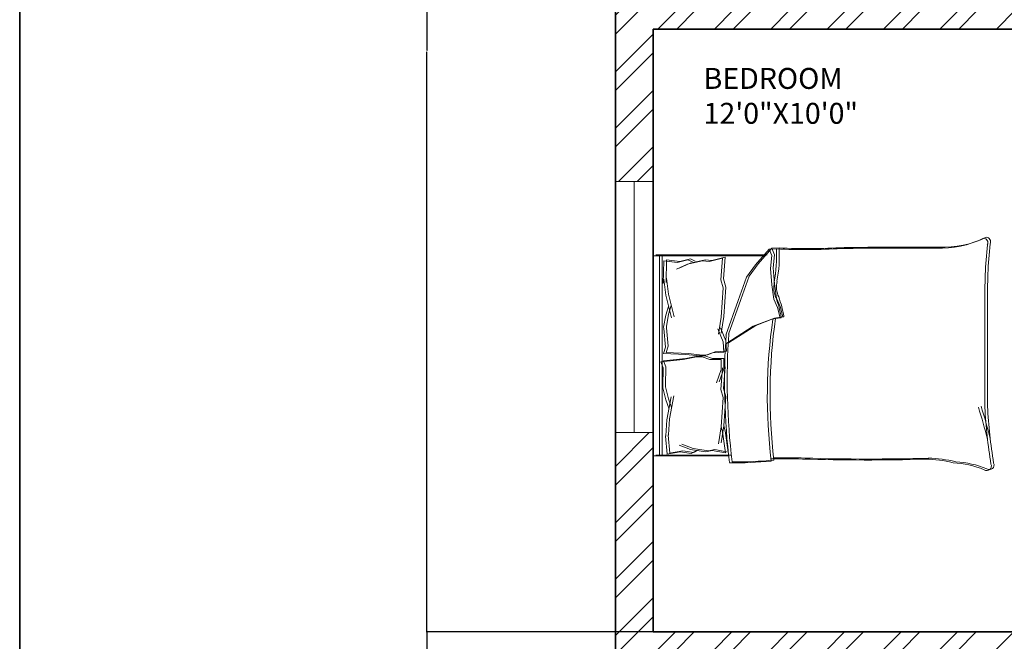
# Model space of a CAD drawing. Units: inches. Extents: x 2120 to 4013, y 1390 to 3019.
# Tile 28 of 59: x 2120 to 2356, y 2073 to 2221. Entities that reach past the tile are written whole.
import ezdxf

# ---------------------------------------------------------------- set-up
doc = ezdxf.new("R2010")
doc.units = ezdxf.units.IN
for name, color, linetype, lineweight in [('A-ANNO-DIMS', 2, 'Continuous', 18), ('A-ANNO-TTLB', 7, 'Continuous', 35), ('A-AREA-IDEN', 7, 'Continuous', 18), ('A-FURN', 8, 'Continuous', 13), ('A-GLAZ', 4, 'Continuous', 18), ('A-WALL', 7, 'Continuous', 35), ('A-WALL-PATT', 252, 'Continuous', 13)]:
    doc.layers.add(name, color=color, linetype=linetype, lineweight=lineweight)
doc.styles.get("Standard").update_dxf_attribs({"font": 'arial.ttf'})
doc.dimstyles.get("Standard").update_dxf_attribs({"dimtxt": 0.18, "dimasz": 0.18, "dimexe": 0.18, "dimexo": 0.0625, "dimgap": 0.09, "dimtad": 0, "dimtih": 1, "dimtoh": 1, "dimdec": 4, "dimzin": 0, "dimdsep": 46, "dimtxsty": 'Standard', "dimcen": 0.09, "dimadec": 0, "dimazin": 0, "dimtfac": 1, "dimtdec": 4, "dimtofl": 0, "dimtmove": 0, "dimatfit": 3, "dimfxl": 1, "dimtolj": 1, "dimtzin": 0, "dimarcsym": 0})

# ---------------------------------------------------------------- blocks, each defined once
blk = doc.blocks.new('BED-DOUBLE-PLAN')
for p, q in [((3.48, 63.34), (3.48, 81.45)), ((3.48, 81.45), (51.27, 81.45)), ((3.7, 62.7), (3.7, 80.81)), ((51.27, 81.45), (51.27, 54.84)), ((51.5, 80.81), (51.5, 54.2)), ((3.48, 79.91), (51.27, 79.91)), ((3.7, 79.27), (51.5, 79.27)), ((3.9, 78.11), (8.18, 78.44)), ((3.9, 78.13), (4.47, 74.95)), ((4.13, 77.47), (8.41, 77.8)), ((8.18, 78.44), (8.29, 78.42)), ((8.29, 78.42), (12.11, 78.13)), ((8.41, 77.8), (8.51, 77.78)), ((8.51, 77.78), (12.34, 77.49)), ((12.11, 78.13), (17.6, 77.12)), ((14.86, 77.7), (16.88, 78.42)), ((15.08, 77.06), (17.11, 77.78)), ((16.88, 78.42), (19.77, 79.14)), ((17.11, 77.78), (20, 78.5)), ((19.77, 79.14), (20.09, 79.14)), ((20, 78.5), (20.32, 78.5)), ((20.09, 79.14), (24.54, 79)), ((20.32, 78.5), (24.77, 78.36)), ((24.54, 79), (25.98, 79.58)), ((24.77, 78.36), (26.21, 78.94)), ((25.98, 79.58), (26.56, 74.23)), ((26.21, 78.94), (26.79, 73.59)), ((27.98, 78.95), (27.73, 73.58)), ((28.21, 78.32), (27.96, 72.94)), ((29.46, 78.47), (27.98, 78.95)), ((29.69, 77.83), (28.21, 78.32)), ((33.89, 78.89), (29.46, 78.47)), ((34.11, 78.25), (29.69, 77.83)), ((34.21, 78.91), (33.89, 78.89)), ((34.43, 78.27), (34.11, 78.25)), ((37.14, 78.37), (34.21, 78.91)), ((37.37, 77.73), (34.43, 78.27)), ((41.92, 78.38), (36.5, 77.02)), ((42.14, 77.74), (36.72, 76.38)), ((39.2, 77.77), (37.14, 78.37)), ((39.43, 77.13), (37.37, 77.73)), ((45.71, 78.9), (41.92, 78.38)), ((45.94, 78.26), (42.14, 77.74)), ((50.11, 78.89), (44.71, 78.99)), ((44.71, 78.99), (45.71, 78.9)), ((50.34, 78.25), (44.94, 78.35)), ((44.94, 78.35), (45.94, 78.26)), ((50.11, 78.89), (49.73, 75.68)), ((50.34, 78.25), (49.96, 75.04)), ((4.12, 77.49), (4.7, 74.31)), ((12.34, 77.49), (17.83, 76.48)), ((49.31, 73.19), (48.13, 75.87)), ((49.73, 75.68), (50.33, 73.11)), ((4.47, 74.95), (4.04, 72.35)), ((4.7, 74.31), (4.27, 71.71)), ((5.05, 72.49), (6.06, 75.24)), ((5.28, 71.85), (6.29, 74.6)), ((26.56, 74.23), (27.14, 71.05)), ((26.79, 73.59), (27.37, 70.41)), ((27.73, 73.58), (27.36, 70.37)), ((27.96, 72.94), (27.58, 69.73)), ((49.54, 72.55), (48.36, 75.23)), ((50.11, 69.62), (49.31, 73.19)), ((50.33, 73.11), (49.82, 72.06)), ((49.96, 75.04), (50.56, 72.47)), ((4.04, 72.35), (4.62, 71.33)), ((4.27, 71.71), (4.85, 70.7)), ((4.47, 68.88), (5.05, 72.49)), ((4.7, 68.24), (5.28, 71.85)), ((27.14, 71.05), (27.14, 69.74)), ((50.34, 68.98), (49.54, 72.55)), ((50.56, 72.47), (50.04, 71.42)), ((4.76, 67.29), (4.47, 68.88)), ((4.99, 66.65), (4.7, 68.24)), ((27.14, 69.74), (26.56, 67.86)), ((27.37, 69.1), (26.79, 67.23)), ((27.36, 70.37), (27.44, 69.07)), ((27.37, 70.41), (27.37, 69.1)), ((27.44, 69.07), (28.13, 67.23)), ((27.58, 69.73), (27.67, 68.43)), ((27.67, 68.43), (28.36, 66.59)), ((49.92, 68.01), (50.11, 69.62)), ((50.15, 67.37), (50.34, 68.98)), ((4.19, 64.11), (4.76, 67.29)), ((4.41, 63.47), (4.99, 66.65)), ((24.1, 65.18), (20.96, 66.27)), ((26.56, 67.86), (26.56, 65.18)), ((26.79, 67.23), (26.79, 64.54)), ((28.13, 67.23), (28.3, 64.55)), ((28.36, 66.59), (28.53, 63.91)), ((30.75, 64.71), (33.82, 65.99)), ((50.7, 64.87), (49.92, 68.01)), ((50.93, 64.23), (50.15, 67.37)), ((9.28, 64.83), (4.19, 64.11)), ((9.51, 64.19), (4.41, 63.47)), ((6.38, 65.82), (10.42, 65.15)), ((6.61, 65.18), (10.64, 64.51)), ((10.42, 65.15), (9.28, 64.83)), ((10.64, 64.51), (9.51, 64.19)), ((10.42, 65.15), (17.43, 64.72)), ((10.64, 64.51), (17.65, 64.08)), ((17.43, 64.72), (19.39, 65.28)), ((17.65, 64.08), (19.61, 64.64)), ((19.39, 65.28), (24.52, 64.87)), ((19.61, 64.64), (24.75, 64.23)), ((24.33, 64.54), (21.19, 65.63)), ((26.56, 65.18), (24.1, 65.18)), ((26.79, 64.54), (24.33, 64.54)), ((28.3, 64.55), (30.75, 64.71)), ((28.53, 63.91), (30.98, 64.07)), ((30.26, 64.06), (34.45, 57.57)), ((30.98, 64.07), (34.05, 65.35)), ((40.65, 61.13), (32.31, 64.06)), ((32.57, 65.82), (36.6, 65.15)), ((32.79, 65.18), (36.83, 64.51)), ((36.6, 65.15), (43.61, 64.72)), ((36.83, 64.51), (43.84, 64.08)), ((43.61, 64.72), (45.57, 65.28)), ((43.84, 64.08), (45.8, 64.64)), ((45.57, 65.28), (50.7, 64.87)), ((45.8, 64.64), (50.93, 64.23)), ((30.49, 63.42), (34.68, 56.93)), ((40.87, 60.49), (32.54, 63.42)), ((46.22, 59.12), (40.65, 61.13)), ((46.45, 58.48), (40.87, 60.49)), ((49.16, 56.95), (46.22, 59.12)), ((34.45, 57.57), (36.15, 53.08)), ((34.68, 56.93), (36.38, 52.44)), ((49.39, 56.31), (46.45, 58.48)), ((52.87, 53.7), (49.16, 56.95)), ((53.1, 53.06), (49.39, 56.31)), ((36.15, 53.08), (36.46, 51.07)), ((36.38, 52.44), (36.69, 50.43)), ((38.94, 51.69), (40.96, 52.62)), ((39.17, 51.05), (41.18, 51.98)), ((40.96, 52.62), (44.36, 53.08)), ((41.18, 51.98), (44.59, 52.44)), ((44.36, 53.08), (48.23, 53.39)), ((44.59, 52.44), (48.46, 52.75)), ((48.23, 53.39), (51.33, 53.08)), ((48.46, 52.75), (51.56, 52.44)), ((51.33, 53.08), (52.87, 53.7)), ((51.56, 52.44), (53.1, 53.06)), ((52.95, 51.96), (52.87, 53.7, 3.87)), ((53.18, 51.32), (53.1, 53.06, 3.87)), ((36.46, 51.07), (38.94, 51.69)), ((36.69, 50.43), (39.17, 51.05)), ((15.06, 2.2), (39.68, 2.2)), ((15.29, 1.56), (39.91, 1.56))]:
    blk.add_line(p, q)
for centre, radius, start, end in [((21.36, -100.61), 164.97, 86.0865, 96.7821), ((21.59, -101.25), 164.97, 86.0865, 96.7821), ((85.16, 61.35), 83.31, 178.7218, 185.604), ((85.39, 60.71), 83.31, 178.7218, 185.604), ((17.76, -74.87), 129.02, 81.7845, 96.9006), ((17.99, -75.51), 129.02, 81.7845, 96.9006), ((-167.31, 50.27), 170.11, 358.4762, 1.0082), ((-167.08, 49.63), 170.11, 358.4762, 1.0082), ((31.16, 79.96), 29.65, 280.6617, 289.8806), ((43.74, 46.38), 6.22, 78.6608, 113.7384), ((43.97, 45.74), 6.22, 78.6608, 113.7384), ((51.33, 88.1), 36.18, 259.8763, 272.5657), ((51.56, 87.46), 36.18, 259.8763, 272.5657), ((182.27, 45.13), 129.5, 176.9791, 183.8365), ((36.64, 51.01), 0.185, 160.2464, 271.1377), ((36.87, 50.37), 0.185, 160.2464, 271.1377), ((31.38, 79.32), 29.65, 280.6617, 289.8806), ((182.5, 44.49), 129.5, 176.9791, 183.8365), ((484.82, 30.83), 482.31, 178.2277, 181.7185), ((485.05, 30.19), 482.31, 178.2277, 181.7185), ((-4508.74, 13.62), 4561.86, 0.00217, 0.28689), ((-4508.51, 12.99), 4561.86, 0.00217, 0.28689), ((-26.9, 16.93), 29.63, 346.0648, 358.9113), ((-26.67, 16.29), 29.63, 346.0648, 358.9113), ((76.16, 12.78), 23.07, 177.4714, 206.4681), ((76.39, 12.14), 23.07, 177.4714, 206.4681), ((-21.66, 11.17), 23.56, 337.9751, 356.652), ((-21.43, 10.53), 23.56, 337.9751, 356.652), ((-17.22, 105.16), 106.46, 283.3832, 287.7053), ((-16.99, 104.52), 106.46, 283.3832, 287.7053), ((54.41, 2.58), 1.1, 242.6588, 356.02), ((1.09, 1.73), 1.09, 146.1736, 293.4781), ((1.32, 1.09), 1.09, 146.1736, 293.4781), ((21.43, -119.39), 121.76, 92.9958, 99.4091), ((21.66, -120.03), 121.76, 92.9958, 99.4091), ((41.15, -130.83), 133.04, 84.4998, 90.6351), ((41.38, -131.47), 133.04, 84.4998, 90.6351), ((54.64, 1.94), 1.1, 242.6588, 356.02)]:
    blk.add_arc(centre, radius, start, end)
blk = doc.blocks.new('WIN-PLAN-60IN')
for p, q in [((0, 9), (0, 0)), ((60, 4.5), (60, 9)), ((60, 9), (60, 0)), ((0, 0), (0, 4.5)), ((0, 4.5), (60, 4.5))]:
    blk.add_line(p, q)
blk = doc.blocks.new('*D214')
at = {"layer": 'A-ANNO-DIMS', "color": 0, "lineweight": -2, "transparency": 16777216}
for p, q in [((2271.67, 2075.03), (2217.55, 2075.03)), ((2217.73, 2074.85), (2217.73, 1970.46)), ((2217.73, 1865.71), (2217.73, 1970.1)), ((2271.67, 1865.53), (2217.55, 1865.53))]:
    blk.add_line(p, q, dxfattribs=at)
at = {"layer": 'A-ANNO-DIMS', "color": 0, "transparency": 16777216}
for points in [[(2217.7, 2074.85), (2217.76, 2074.85), (2217.73, 2075.03)], [(2217.7, 1865.71), (2217.76, 1865.71), (2217.73, 1865.53)]]:
    blk.add_solid(points, dxfattribs=at)
at = {"layer": 'Defpoints', "color": 0, "transparency": 16777216}
for p in [(2217.73, 2075.03), (2271.73, 2075.03), (2271.73, 1865.53)]:
    blk.add_point(p, dxfattribs=at)
at = {"layer": 'A-ANNO-DIMS', "color": 0, "transparency": 16777216, "insert": (2217.73, 1970.28), "char_height": 0.18, "attachment_point": 5}
blk.add_mtext('\\A1;209.5', dxfattribs=at)
blk = doc.blocks.new('*D215')
at = {"layer": 'A-ANNO-DIMS', "color": 0, "lineweight": -2, "transparency": 16777216}
for p, q in [((2262.67, 2352.53), (2217.55, 2352.53)), ((2217.73, 2352.35), (2217.73, 2213.96)), ((2217.73, 2075.21), (2217.73, 2213.6)), ((2271.67, 2075.03), (2217.55, 2075.03))]:
    blk.add_line(p, q, dxfattribs=at)
at = {"layer": 'A-ANNO-DIMS', "color": 0, "transparency": 16777216}
for points in [[(2217.7, 2352.35), (2217.76, 2352.35), (2217.73, 2352.53)], [(2217.7, 2075.21), (2217.76, 2075.21), (2217.73, 2075.03)]]:
    blk.add_solid(points, dxfattribs=at)
at = {"layer": 'Defpoints', "color": 0, "transparency": 16777216}
for p in [(2217.73, 2352.53), (2262.73, 2352.53), (2271.73, 2075.03)]:
    blk.add_point(p, dxfattribs=at)
at = {"layer": 'A-ANNO-DIMS', "color": 0, "transparency": 16777216, "insert": (2217.73, 2213.78), "char_height": 0.18, "attachment_point": 5}
blk.add_mtext('\\A1;277.5', dxfattribs=at)

msp = doc.modelspace()

# ---------------------------------------------------------------- hatches: boundary and pattern name
at = {"layer": 'A-WALL-PATT'}
h = msp.add_hatch(dxfattribs=at)
h.set_pattern_fill('ANSI32', color=256)
h.paths.add_polyline_path([(2271.7331, 2343.531), (2283.3788, 2343.531), (2283.3788, 2348.031), (2283.3788, 2352.5306), (2262.7331, 2352.5306), (2262.7331, 2182.638), (2267.2331, 2182.638), (2271.7331, 2182.638), (2271.7331, 2219.031), (2391.7331, 2219.031), (2391.7331, 2214.189), (2393.9831, 2214.189), (2396.2331, 2214.189), (2396.2331, 2219.031), (2420.2331, 2219.031), (2420.2331, 2225.7535), (2417.2197, 2225.7535), (2415.7331, 2225.7535), (2415.7331, 2223.5306), (2271.7331, 2223.5306)])
h.paths.add_polyline_path([(2380.0942, 2352.5306), (2343.3788, 2352.5306), (2343.3788, 2343.531), (2363.2331, 2343.531), (2363.2331, 2288.8489), (2365.4831, 2288.8489), (2367.7331, 2288.8489), (2367.7331, 2343.531), (2380.0942, 2343.531)], flags=17)
h.paths.add_polyline_path([(2432.4339, 2352.5306), (2404.0943, 2352.5306), (2404.0943, 2343.531), (2415.7331, 2343.531), (2415.7331, 2264.0306), (2367.7331, 2264.0306), (2367.7331, 2266.4872), (2363.2331, 2266.4872), (2363.2331, 2259.531), (2367.7331, 2259.531), (2415.7331, 2259.531), (2415.7331, 2255.0658), (2420.2331, 2255.0658), (2420.2331, 2259.531), (2424.5717, 2259.531), (2424.5717, 2261.781), (2424.5717, 2264.0306), (2420.2331, 2264.0306), (2420.2331, 2343.531), (2432.4339, 2343.531)])
h.paths.add_polyline_path([(2508.9115, 2352.5306), (2456.4339, 2352.5306), (2456.4339, 2343.531), (2468.2331, 2343.531), (2468.2331, 2264.0306), (2448.0487, 2264.0306), (2448.0487, 2259.531), (2468.2331, 2259.531), (2468.2331, 2255.5496), (2472.7331, 2255.5496), (2472.7331, 2343.531), (2508.9115, 2343.531)])
h.paths.add_polyline_path([(2637.7331, 2352.5306), (2544.9116, 2352.5306), (2544.9116, 2343.531), (2589.7331, 2343.531), (2633.2331, 2343.531), (2637.7331, 2343.531)])
h.paths.add_polyline_path([(2594.2331, 2343.5306), (2589.7331, 2343.5306), (2589.7331, 2259.5306), (2589.7331, 2252.4915), (2591.9831, 2252.4915), (2594.2331, 2252.4915)])
h.paths.add_polyline_path([(2637.7331, 2223.5306), (2594.2331, 2223.5306), (2594.2331, 2230.1988), (2591.9831, 2230.1988), (2589.7331, 2230.1988), (2589.7331, 2223.5306), (2472.7331, 2223.5306), (2468.2331, 2223.5306), (2468.2331, 2219.031), (2628.7331, 2219.031), (2628.7331, 2138.031), (2637.7331, 2138.031)])
h.paths.add_polyline_path([(3822.6535, 2458.4402), (3874.9468, 2458.4402), (3874.9468, 2476.9866), (3822.6535, 2476.9866)], flags=9)
h.paths.add_polyline_path([(3834.6921, 2781.8174), (3935.9206, 2781.8174), (3935.9206, 2800.3638), (3834.6921, 2800.3638)], flags=9)
h.paths.add_polyline_path([(3832.2843, 2837.9683), (3884.5776, 2837.9683), (3884.5776, 2856.5146), (3832.2843, 2856.5146)], flags=9)
h.paths.add_polyline_path([(3830.9388, 2861.4782), (3956.8958, 2861.4782), (3956.8958, 2880.0245), (3830.9388, 2880.0245)], flags=9)
h.paths.add_polyline_path([(3870.6966, 2352.5752), (3887.9272, 2352.5752), (3887.9272, 2377.3037), (3870.6966, 2377.3037)], flags=9)
h.paths.add_polyline_path([(3289.2701, 2413.161), (3435.2223, 2413.161), (3435.2223, 2450.2538), (3289.2701, 2450.2538)], flags=9)
h.paths.add_polyline_path([(2487.6944, 2414.3601), (2637.8335, 2414.3601), (2637.8335, 2451.4528), (2487.6944, 2451.4528)], flags=9)
h.paths.add_polyline_path([(2567.3724, 1457.9199), (2815.296, 1457.9199), (2815.296, 1495.0127), (2567.3724, 1495.0127)], flags=9)
h.paths.add_polyline_path([(2655.3825, 2093.2363), (2685.9555, 2093.2363), (2685.9555, 2111.8937), (2655.3825, 2111.8937)], flags=9)
h.paths.add_polyline_path([(2543.9218, 1550.6671), (2587.8406, 1550.6671), (2587.8406, 1569.3244), (2543.9218, 1569.3244)], flags=9)
h.paths.add_polyline_path([(2905.1384, 1543.8113), (2949.0572, 1543.8113), (2949.0572, 1562.4686), (2905.1384, 1562.4686)], flags=9)
h.paths.add_polyline_path([(2736.4118, 1702.4736), (2784.2153, 1702.4736), (2784.2153, 1721.1309), (2736.4118, 1721.1309)], flags=9)
h.paths.add_polyline_path([(2912.8666, 1710.4168), (2951.707, 1710.4168), (2951.707, 1729.0741), (2912.8666, 1729.0741)], flags=9)
h.paths.add_polyline_path([(2923.5785, 1763.5038), (2959.7279, 1763.5038), (2959.7279, 1782.1611), (2923.5785, 1782.1611)], flags=9)
h.paths.add_polyline_path([(2925.2114, 1809.6137), (2967.1861, 1809.6137), (2967.1861, 1828.271), (2925.2114, 1828.271)], flags=9)
h.paths.add_polyline_path([(2996.2711, 1878.9003), (2996.2711, 1913.109), (2977.6138, 1913.109), (2977.6138, 1878.9003)], flags=9)
h.paths.add_polyline_path([(2883.0859, 1895.7192), (2927.1855, 1895.7192), (2927.1855, 1914.3766), (2883.0859, 1914.3766)], flags=9)
h.paths.add_polyline_path([(2787.3924, 1810.8013), (2841.0213, 1810.8013), (2841.0213, 1829.4587), (2787.3924, 1829.4587)], flags=9)
h.paths.add_polyline_path([(2775.6399, 2101.7395), (2829.2689, 2101.7395), (2829.2689, 2120.3968), (2775.6399, 2120.3968)], flags=9)
h.paths.add_polyline_path([(2913.0263, 2075.817), (2951.8667, 2075.817), (2951.8667, 2094.4744), (2913.0263, 2094.4744)], flags=9)
h.paths.add_polyline_path([(2929.966, 2133.3669), (2966.1154, 2133.3669), (2966.1154, 2152.0243), (2929.966, 2152.0243)], flags=9)
h.paths.add_polyline_path([(2932.7502, 2182.6088), (2968.8996, 2182.6088), (2968.8996, 2201.2662), (2932.7502, 2201.2662)], flags=9)
h.paths.add_polyline_path([(2996.0681, 2266.3173), (2996.0681, 2300.5261), (2977.4108, 2300.5261), (2977.4108, 2266.3173)], flags=9)
h.paths.add_polyline_path([(2885.1039, 2279.2186), (2929.2035, 2279.2186), (2929.2035, 2297.8759), (2885.1039, 2297.8759)], flags=9)
h.paths.add_polyline_path([(2735.7042, 2218.3197), (2783.5078, 2218.3197), (2783.5078, 2236.9771), (2735.7042, 2236.9771)], flags=9)
h.paths.add_polyline_path([(2635.6049, 2044.0085), (2648.9678, 2044.0085), (2648.9678, 2054.312), (2635.6049, 2054.312)], flags=9)
h.paths.add_polyline_path([(2714.0148, 1923.0473), (2727.3777, 1923.0473), (2727.3777, 1933.3508), (2714.0148, 1933.3508)], flags=9)
h.paths.add_polyline_path([(2709.0345, 1988.1628), (2722.3974, 1988.1628), (2722.3974, 1998.4663), (2709.0345, 1998.4663)], flags=9)
h.paths.add_polyline_path([(2592.8935, 1962.1763), (2606.2564, 1962.1763), (2606.2564, 1972.4799), (2592.8935, 1972.4799)], flags=9)
h.paths.add_polyline_path([(2618.3996, 1985.9724), (2644.1942, 1985.9724), (2644.1942, 1996.2759), (2618.3996, 1996.2759)], flags=9)
h.paths.add_polyline_path([(2601.279, 1920.5869), (2614.6419, 1920.5869), (2614.6419, 1930.8904), (2601.279, 1930.8904)], flags=9)
h.paths.add_polyline_path([(2692.3278, 1932.7645), (2704.5311, 1932.7645), (2704.5311, 1943.0681), (2692.3278, 1943.0681)], flags=9)
h.paths.add_polyline_path([(2311.122, 1672.7318), (2355.0408, 1672.7318), (2355.0408, 1691.3892), (2311.122, 1691.3892)], flags=9)
h.paths.add_polyline_path([(2456.2551, 1632.3198), (2492.4796, 1632.3198), (2492.4796, 1650.9772), (2456.2551, 1650.9772)], flags=9)
h.paths.add_polyline_path([(2401.0766, 1631.4793), (2437.301, 1631.4793), (2437.301, 1650.1367), (2401.0766, 1650.1367)], flags=9)
h.paths.add_polyline_path([(2546.7054, 1700.9235), (2594.509, 1700.9235), (2594.509, 1719.5809), (2546.7054, 1719.5809)], flags=9)
h.paths.add_polyline_path([(2445.4866, 1766.9937), (2497.5261, 1766.9937), (2497.5261, 1785.651), (2445.4866, 1785.651)], flags=9)
h.paths.add_polyline_path([(2287.9992, 1739.7675), (2326.8396, 1739.7675), (2326.8396, 1758.4248), (2287.9992, 1758.4248)], flags=9)
h.paths.add_polyline_path([(2458.5279, 1924.7607), (2510.5675, 1924.7607), (2510.5675, 1943.4181), (2458.5279, 1943.4181)], flags=9)
h.paths.add_polyline_path([(2309.2811, 1902.7642), (2345.4305, 1902.7642), (2345.4305, 1921.4215), (2309.2811, 1921.4215)], flags=9)
h.paths.add_polyline_path([(2490.7554, 2018.9392), (2530.7896, 2018.9392), (2530.7896, 2037.5965), (2490.7554, 2037.5965)], flags=9)
h.paths.add_polyline_path([(2402.143, 2024.7393), (2438.5414, 2024.7393), (2438.5414, 2043.3966), (2402.143, 2043.3966)], flags=9)
h.paths.add_polyline_path([(2287.856, 1931.7926), (2326.6964, 1931.7926), (2326.6964, 1950.4499), (2287.856, 1950.4499)], flags=9)
h.paths.add_polyline_path([(2281.7979, 2193.5771), (2320.6383, 2193.5771), (2320.6383, 2212.2344), (2281.7979, 2212.2344)], flags=25)
h.paths.add_polyline_path([(2484.0754, 2093.892), (2536.115, 2093.892), (2536.115, 2112.5494), (2484.0754, 2112.5494)], flags=9)
h.paths.add_polyline_path([(2624.7948, 2281.8639), (2624.7948, 2311.4137), (2606.1375, 2311.4137), (2606.1375, 2281.8639)], flags=9)
h.paths.add_polyline_path([(2507.5036, 2290.3639), (2541.934, 2290.3639), (2541.934, 2309.0212), (2507.5036, 2309.0212)], flags=9)
h.paths.add_polyline_path([(2423.1076, 2285.2202), (2459.332, 2285.2202), (2459.332, 2303.8776), (2423.1076, 2303.8776)], flags=9)
h.paths.add_polyline_path([(2374.5467, 2289.6272), (2410.7711, 2289.6272), (2410.7711, 2308.2846), (2374.5467, 2308.2846)], flags=25)
h.paths.add_polyline_path([(2277.4907, 2227.5651), (2316.3311, 2227.5651), (2316.3311, 2246.2224), (2277.4907, 2246.2224)], flags=25)
h.paths.add_polyline_path([(2655.3825, 2093.2367), (2685.9555, 2093.2367), (2685.9555, 2111.894), (2655.3825, 2111.894)], flags=9)
h.paths.add_polyline_path([(2543.9217, 1550.6674), (2587.8406, 1550.6674), (2587.8406, 1569.3247), (2543.9217, 1569.3247)], flags=9)
h.paths.add_polyline_path([(2905.1384, 1543.8116), (2949.0572, 1543.8116), (2949.0572, 1562.4689), (2905.1384, 1562.4689)], flags=9)
h.paths.add_polyline_path([(2736.4118, 1702.4739), (2784.2153, 1702.4739), (2784.2153, 1721.1312), (2736.4118, 1721.1312)], flags=9)
h.paths.add_polyline_path([(2912.8666, 1710.4171), (2951.707, 1710.4171), (2951.707, 1729.0744), (2912.8666, 1729.0744)], flags=9)
h.paths.add_polyline_path([(2923.5785, 1763.5041), (2959.7279, 1763.5041), (2959.7279, 1782.1614), (2923.5785, 1782.1614)], flags=9)
h.paths.add_polyline_path([(2925.2114, 1809.614), (2967.1861, 1809.614), (2967.1861, 1828.2713), (2925.2114, 1828.2713)], flags=9)
h.paths.add_polyline_path([(2996.2711, 1878.9006), (2996.2711, 1913.1094), (2977.6137, 1913.1094), (2977.6137, 1878.9006)], flags=9)
h.paths.add_polyline_path([(2883.0859, 1895.7195), (2927.1855, 1895.7195), (2927.1855, 1914.3769), (2883.0859, 1914.3769)], flags=9)
h.paths.add_polyline_path([(2787.3924, 1810.8016), (2841.0213, 1810.8016), (2841.0213, 1829.459), (2787.3924, 1829.459)], flags=9)
h.paths.add_polyline_path([(2775.6399, 2101.7398), (2829.2688, 2101.7398), (2829.2688, 2120.3971), (2775.6399, 2120.3971)], flags=9)
h.paths.add_polyline_path([(2913.0263, 2075.8173), (2951.8667, 2075.8173), (2951.8667, 2094.4747), (2913.0263, 2094.4747)], flags=9)
h.paths.add_polyline_path([(2929.966, 2133.3672), (2966.1154, 2133.3672), (2966.1154, 2152.0246), (2929.966, 2152.0246)], flags=9)
h.paths.add_polyline_path([(2932.7502, 2182.6091), (2968.8996, 2182.6091), (2968.8996, 2201.2665), (2932.7502, 2201.2665)], flags=9)
h.paths.add_polyline_path([(2996.0681, 2266.3176), (2996.0681, 2300.5264), (2977.4108, 2300.5264), (2977.4108, 2266.3176)], flags=9)
h.paths.add_polyline_path([(2885.1039, 2279.2189), (2929.2035, 2279.2189), (2929.2035, 2297.8762), (2885.1039, 2297.8762)], flags=9)
h.paths.add_polyline_path([(2735.7042, 2218.32), (2783.5078, 2218.32), (2783.5078, 2236.9774), (2735.7042, 2236.9774)], flags=9)
h.paths.add_polyline_path([(2635.6048, 2044.0088), (2648.9677, 2044.0088), (2648.9677, 2054.3123), (2635.6048, 2054.3123)], flags=9)
h.paths.add_polyline_path([(2714.0148, 1923.0476), (2727.3777, 1923.0476), (2727.3777, 1933.3511), (2714.0148, 1933.3511)], flags=9)
h.paths.add_polyline_path([(2709.0345, 1988.1631), (2722.3974, 1988.1631), (2722.3974, 1998.4666), (2709.0345, 1998.4666)], flags=9)
h.paths.add_polyline_path([(2592.8935, 1962.1766), (2606.2564, 1962.1766), (2606.2564, 1972.4802), (2592.8935, 1972.4802)], flags=9)
h.paths.add_polyline_path([(2618.3995, 1985.9727), (2644.1942, 1985.9727), (2644.1942, 1996.2762), (2618.3995, 1996.2762)], flags=9)
h.paths.add_polyline_path([(2601.279, 1920.5872), (2614.6419, 1920.5872), (2614.6419, 1930.8908), (2601.279, 1930.8908)], flags=9)
h.paths.add_polyline_path([(2692.3278, 1932.7648), (2704.5311, 1932.7648), (2704.5311, 1943.0684), (2692.3278, 1943.0684)], flags=9)
h.paths.add_polyline_path([(2311.122, 1672.7321), (2355.0408, 1672.7321), (2355.0408, 1691.3895), (2311.122, 1691.3895)], flags=9)
h.paths.add_polyline_path([(2456.2551, 1632.3201), (2492.4795, 1632.3201), (2492.4795, 1650.9775), (2456.2551, 1650.9775)], flags=9)
h.paths.add_polyline_path([(2401.0766, 1631.4796), (2437.301, 1631.4796), (2437.301, 1650.137), (2401.0766, 1650.137)], flags=9)
h.paths.add_polyline_path([(2546.7054, 1700.9238), (2594.509, 1700.9238), (2594.509, 1719.5812), (2546.7054, 1719.5812)], flags=9)
h.paths.add_polyline_path([(2445.4866, 1766.994), (2497.5261, 1766.994), (2497.5261, 1785.6513), (2445.4866, 1785.6513)], flags=9)
h.paths.add_polyline_path([(2287.9992, 1739.7678), (2326.8396, 1739.7678), (2326.8396, 1758.4251), (2287.9992, 1758.4251)], flags=9)
h.paths.add_polyline_path([(2458.5279, 1924.7611), (2510.5675, 1924.7611), (2510.5675, 1943.4184), (2458.5279, 1943.4184)], flags=9)
h.paths.add_polyline_path([(2309.2811, 1902.7645), (2345.4305, 1902.7645), (2345.4305, 1921.4218), (2309.2811, 1921.4218)], flags=9)
h.paths.add_polyline_path([(2490.7554, 2018.9395), (2530.7895, 2018.9395), (2530.7895, 2037.5968), (2490.7554, 2037.5968)], flags=9)
h.paths.add_polyline_path([(2402.143, 2024.7396), (2438.5413, 2024.7396), (2438.5413, 2043.3969), (2402.143, 2043.3969)], flags=9)
h.paths.add_polyline_path([(2287.856, 1931.7929), (2326.6964, 1931.7929), (2326.6964, 1950.4502), (2287.856, 1950.4502)], flags=9)
h.paths.add_polyline_path([(2281.7979, 2193.5774), (2320.6383, 2193.5774), (2320.6383, 2212.2347), (2281.7979, 2212.2347)], flags=25)
h.paths.add_polyline_path([(2484.0754, 2093.8924), (2536.115, 2093.8924), (2536.115, 2112.5497), (2484.0754, 2112.5497)], flags=9)
h.paths.add_polyline_path([(2624.7948, 2281.8642), (2624.7948, 2311.414), (2606.1374, 2311.414), (2606.1374, 2281.8642)], flags=9)
h.paths.add_polyline_path([(2507.5035, 2290.3642), (2541.934, 2290.3642), (2541.934, 2309.0215), (2507.5035, 2309.0215)], flags=9)
h.paths.add_polyline_path([(2423.1075, 2285.2205), (2459.332, 2285.2205), (2459.332, 2303.8779), (2423.1075, 2303.8779)], flags=9)
h.paths.add_polyline_path([(2374.5467, 2289.6275), (2410.7711, 2289.6275), (2410.7711, 2308.2849), (2374.5467, 2308.2849)], flags=25)
h.paths.add_polyline_path([(2277.4907, 2227.5654), (2316.3311, 2227.5654), (2316.3311, 2246.2227), (2277.4907, 2246.2227)], flags=25)
h = msp.add_hatch(dxfattribs=at)
h.set_pattern_fill('ANSI32', color=256)
h.paths.add_polyline_path([(2271.7331, 1980.389), (2262.7331, 1980.389), (2262.7331, 1912.8434), (2267.2331, 1912.8434), (2271.7331, 1912.8434), (2271.7331, 1922.531), (2351.2331, 1922.531), (2351.2331, 1901.4728), (2355.7331, 1901.4728), (2355.7331, 1922.531), (2357.9815, 1922.531), (2357.9815, 1926.5306), (2271.7331, 1926.5306)])
h.paths.add_polyline_path([(2589.2331, 1949.1622), (2584.7331, 1949.1622), (2580.2331, 1949.1622), (2580.2331, 1874.5306), (2355.7331, 1874.5306), (2355.7331, 1880.1922), (2351.2331, 1880.1922), (2351.2331, 1874.5306), (2271.7331, 1874.5306), (2271.7331, 1888.8431), (2262.7331, 1888.8431), (2262.7331, 1842.2909), (2267.2331, 1842.2909), (2271.7331, 1842.2909), (2271.7331, 1865.531), (2415.7331, 1865.531), (2415.7331, 1779.7286), (2420.2331, 1779.7286), (2420.2331, 1865.531), (2589.2331, 1865.531)])
h.paths.add_polyline_path([(2271.7331, 1782.2906), (2262.7331, 1782.2906), (2262.7331, 1711.4639), (2267.2331, 1711.4639), (2271.7331, 1711.4639), (2271.7331, 1738.031), (2420.2331, 1738.031), (2420.2331, 1742.531), (2420.2331, 1747.3376), (2417.9831, 1747.3376), (2415.7331, 1747.3376), (2415.7331, 1742.5306), (2271.7331, 1742.5306)])
h.paths.add_polyline_path([(2271.7331, 1627.031), (2362.3957, 1627.031), (2362.3957, 1629.281), (2362.3957, 1631.5306), (2271.7331, 1631.5306), (2271.7331, 1675.4636), (2262.7331, 1675.4636), (2262.7331, 1581.531), (2405.3032, 1581.531), (2405.3032, 1586.031), (2405.3032, 1590.5306), (2396.2331, 1590.5306), (2396.2331, 1691.4513), (2418.7206, 1691.4513), (2418.7206, 1695.951), (2396.2331, 1695.951), (2391.7331, 1695.951), (2391.7331, 1631.5306), (2386.7425, 1631.5306), (2386.7425, 1629.2806), (2386.7425, 1627.031), (2391.7331, 1627.031), (2391.7331, 1586.1709), (2271.7331, 1586.1709)])
h.paths.add_polyline_path([(2459.6703, 1590.5306), (2429.3032, 1590.5306), (2429.3032, 1581.531), (2459.6703, 1581.531), (2459.6703, 1586.031)])
h.paths.add_polyline_path([(2501.2331, 1590.531), (2501.2331, 1665.0195), (2498.9831, 1665.0195), (2496.7331, 1665.0195), (2496.7331, 1590.5306), (2483.8201, 1590.5306), (2483.8201, 1590.1579), (2483.6704, 1590.1579), (2483.6704, 1581.531), (2505.0196, 1581.531), (2505.0196, 1583.781), (2505.0196, 1586.0306), (2501.2331, 1586.0306)])
h.paths.add_polyline_path([(2544.1361, 1583.781), (2544.1361, 1586.0306), (2527.1368, 1586.0306), (2527.1368, 1583.7806), (2527.1368, 1581.531), (2544.1361, 1581.531)])
h.paths.add_polyline_path([(3822.6535, 2458.4402), (3874.9468, 2458.4402), (3874.9468, 2476.9866), (3822.6535, 2476.9866)], flags=9)
h.paths.add_polyline_path([(3834.6921, 2781.8174), (3935.9206, 2781.8174), (3935.9206, 2800.3638), (3834.6921, 2800.3638)], flags=9)
h.paths.add_polyline_path([(3832.2843, 2837.9683), (3884.5776, 2837.9683), (3884.5776, 2856.5146), (3832.2843, 2856.5146)], flags=9)
h.paths.add_polyline_path([(3830.9388, 2861.4782), (3956.8958, 2861.4782), (3956.8958, 2880.0245), (3830.9388, 2880.0245)], flags=9)
h.paths.add_polyline_path([(3870.6966, 2352.5752), (3887.9272, 2352.5752), (3887.9272, 2377.3037), (3870.6966, 2377.3037)], flags=9)
h.paths.add_polyline_path([(3289.2701, 2413.161), (3435.2223, 2413.161), (3435.2223, 2450.2538), (3289.2701, 2450.2538)], flags=9)
h.paths.add_polyline_path([(2487.6944, 2414.3601), (2637.8335, 2414.3601), (2637.8335, 2451.4528), (2487.6944, 2451.4528)], flags=9)
h.paths.add_polyline_path([(2567.3724, 1457.9199), (2815.296, 1457.9199), (2815.296, 1495.0127), (2567.3724, 1495.0127)], flags=9)
h.paths.add_polyline_path([(2655.3825, 2093.2363), (2685.9555, 2093.2363), (2685.9555, 2111.8937), (2655.3825, 2111.8937)], flags=9)
h.paths.add_polyline_path([(2543.9218, 1550.6671), (2587.8406, 1550.6671), (2587.8406, 1569.3244), (2543.9218, 1569.3244)], flags=9)
h.paths.add_polyline_path([(2905.1384, 1543.8113), (2949.0572, 1543.8113), (2949.0572, 1562.4686), (2905.1384, 1562.4686)], flags=9)
h.paths.add_polyline_path([(2736.4118, 1702.4736), (2784.2153, 1702.4736), (2784.2153, 1721.1309), (2736.4118, 1721.1309)], flags=9)
h.paths.add_polyline_path([(2912.8666, 1710.4168), (2951.707, 1710.4168), (2951.707, 1729.0741), (2912.8666, 1729.0741)], flags=9)
h.paths.add_polyline_path([(2923.5785, 1763.5038), (2959.7279, 1763.5038), (2959.7279, 1782.1611), (2923.5785, 1782.1611)], flags=9)
h.paths.add_polyline_path([(2925.2114, 1809.6137), (2967.1861, 1809.6137), (2967.1861, 1828.271), (2925.2114, 1828.271)], flags=9)
h.paths.add_polyline_path([(2996.2711, 1878.9003), (2996.2711, 1913.109), (2977.6138, 1913.109), (2977.6138, 1878.9003)], flags=9)
h.paths.add_polyline_path([(2883.0859, 1895.7192), (2927.1855, 1895.7192), (2927.1855, 1914.3766), (2883.0859, 1914.3766)], flags=9)
h.paths.add_polyline_path([(2787.3924, 1810.8013), (2841.0213, 1810.8013), (2841.0213, 1829.4587), (2787.3924, 1829.4587)], flags=9)
h.paths.add_polyline_path([(2775.6399, 2101.7395), (2829.2689, 2101.7395), (2829.2689, 2120.3968), (2775.6399, 2120.3968)], flags=9)
h.paths.add_polyline_path([(2913.0263, 2075.817), (2951.8667, 2075.817), (2951.8667, 2094.4744), (2913.0263, 2094.4744)], flags=9)
h.paths.add_polyline_path([(2929.966, 2133.3669), (2966.1154, 2133.3669), (2966.1154, 2152.0243), (2929.966, 2152.0243)], flags=9)
h.paths.add_polyline_path([(2932.7502, 2182.6088), (2968.8996, 2182.6088), (2968.8996, 2201.2662), (2932.7502, 2201.2662)], flags=9)
h.paths.add_polyline_path([(2996.0681, 2266.3173), (2996.0681, 2300.5261), (2977.4108, 2300.5261), (2977.4108, 2266.3173)], flags=9)
h.paths.add_polyline_path([(2885.1039, 2279.2186), (2929.2035, 2279.2186), (2929.2035, 2297.8759), (2885.1039, 2297.8759)], flags=9)
h.paths.add_polyline_path([(2735.7042, 2218.3197), (2783.5078, 2218.3197), (2783.5078, 2236.9771), (2735.7042, 2236.9771)], flags=9)
h.paths.add_polyline_path([(2635.6049, 2044.0085), (2648.9678, 2044.0085), (2648.9678, 2054.312), (2635.6049, 2054.312)], flags=9)
h.paths.add_polyline_path([(2714.0148, 1923.0473), (2727.3777, 1923.0473), (2727.3777, 1933.3508), (2714.0148, 1933.3508)], flags=9)
h.paths.add_polyline_path([(2709.0345, 1988.1628), (2722.3974, 1988.1628), (2722.3974, 1998.4663), (2709.0345, 1998.4663)], flags=9)
h.paths.add_polyline_path([(2592.8935, 1962.1763), (2606.2564, 1962.1763), (2606.2564, 1972.4799), (2592.8935, 1972.4799)], flags=9)
h.paths.add_polyline_path([(2618.3996, 1985.9724), (2644.1942, 1985.9724), (2644.1942, 1996.2759), (2618.3996, 1996.2759)], flags=9)
h.paths.add_polyline_path([(2601.279, 1920.5869), (2614.6419, 1920.5869), (2614.6419, 1930.8904), (2601.279, 1930.8904)], flags=9)
h.paths.add_polyline_path([(2692.3278, 1932.7645), (2704.5311, 1932.7645), (2704.5311, 1943.0681), (2692.3278, 1943.0681)], flags=9)
h.paths.add_polyline_path([(2311.122, 1672.7318), (2355.0408, 1672.7318), (2355.0408, 1691.3892), (2311.122, 1691.3892)], flags=25)
h.paths.add_polyline_path([(2456.2551, 1632.3198), (2492.4796, 1632.3198), (2492.4796, 1650.9772), (2456.2551, 1650.9772)], flags=9)
h.paths.add_polyline_path([(2401.0766, 1631.4793), (2437.301, 1631.4793), (2437.301, 1650.1367), (2401.0766, 1650.1367)], flags=9)
h.paths.add_polyline_path([(2546.7054, 1700.9235), (2594.509, 1700.9235), (2594.509, 1719.5809), (2546.7054, 1719.5809)], flags=9)
h.paths.add_polyline_path([(2445.4866, 1766.9937), (2497.5261, 1766.9937), (2497.5261, 1785.651), (2445.4866, 1785.651)], flags=9)
h.paths.add_polyline_path([(2287.9992, 1739.7675), (2326.8396, 1739.7675), (2326.8396, 1758.4248), (2287.9992, 1758.4248)], flags=24)
h.paths.add_polyline_path([(2458.5279, 1924.7607), (2510.5675, 1924.7607), (2510.5675, 1943.4181), (2458.5279, 1943.4181)], flags=25)
h.paths.add_polyline_path([(2309.2811, 1902.7642), (2345.4305, 1902.7642), (2345.4305, 1921.4215), (2309.2811, 1921.4215)], flags=25)
h.paths.add_polyline_path([(2490.7554, 2018.9392), (2530.7896, 2018.9392), (2530.7896, 2037.5965), (2490.7554, 2037.5965)], flags=9)
h.paths.add_polyline_path([(2402.143, 2024.7393), (2438.5414, 2024.7393), (2438.5414, 2043.3966), (2402.143, 2043.3966)], flags=9)
h.paths.add_polyline_path([(2287.856, 1931.7926), (2326.6964, 1931.7926), (2326.6964, 1950.4499), (2287.856, 1950.4499)], flags=25)
h.paths.add_polyline_path([(2281.7979, 2193.5771), (2320.6383, 2193.5771), (2320.6383, 2212.2344), (2281.7979, 2212.2344)], flags=9)
h.paths.add_polyline_path([(2484.0754, 2093.892), (2536.115, 2093.892), (2536.115, 2112.5494), (2484.0754, 2112.5494)], flags=9)
h.paths.add_polyline_path([(2624.7948, 2281.8639), (2624.7948, 2311.4137), (2606.1375, 2311.4137), (2606.1375, 2281.8639)], flags=9)
h.paths.add_polyline_path([(2507.5036, 2290.3639), (2541.934, 2290.3639), (2541.934, 2309.0212), (2507.5036, 2309.0212)], flags=9)
h.paths.add_polyline_path([(2423.1076, 2285.2202), (2459.332, 2285.2202), (2459.332, 2303.8776), (2423.1076, 2303.8776)], flags=9)
h.paths.add_polyline_path([(2374.5467, 2289.6272), (2410.7711, 2289.6272), (2410.7711, 2308.2846), (2374.5467, 2308.2846)], flags=9)
h.paths.add_polyline_path([(2277.4907, 2227.5651), (2316.3311, 2227.5651), (2316.3311, 2246.2224), (2277.4907, 2246.2224)], flags=9)
h.paths.add_polyline_path([(2655.3825, 2093.2367), (2685.9555, 2093.2367), (2685.9555, 2111.894), (2655.3825, 2111.894)], flags=9)
h.paths.add_polyline_path([(2543.9217, 1550.6674), (2587.8406, 1550.6674), (2587.8406, 1569.3247), (2543.9217, 1569.3247)], flags=9)
h.paths.add_polyline_path([(2905.1384, 1543.8116), (2949.0572, 1543.8116), (2949.0572, 1562.4689), (2905.1384, 1562.4689)], flags=9)
h.paths.add_polyline_path([(2736.4118, 1702.4739), (2784.2153, 1702.4739), (2784.2153, 1721.1312), (2736.4118, 1721.1312)], flags=9)
h.paths.add_polyline_path([(2912.8666, 1710.4171), (2951.707, 1710.4171), (2951.707, 1729.0744), (2912.8666, 1729.0744)], flags=9)
h.paths.add_polyline_path([(2923.5785, 1763.5041), (2959.7279, 1763.5041), (2959.7279, 1782.1614), (2923.5785, 1782.1614)], flags=9)
h.paths.add_polyline_path([(2925.2114, 1809.614), (2967.1861, 1809.614), (2967.1861, 1828.2713), (2925.2114, 1828.2713)], flags=9)
h.paths.add_polyline_path([(2996.2711, 1878.9006), (2996.2711, 1913.1094), (2977.6137, 1913.1094), (2977.6137, 1878.9006)], flags=9)
h.paths.add_polyline_path([(2883.0859, 1895.7195), (2927.1855, 1895.7195), (2927.1855, 1914.3769), (2883.0859, 1914.3769)], flags=9)
h.paths.add_polyline_path([(2787.3924, 1810.8016), (2841.0213, 1810.8016), (2841.0213, 1829.459), (2787.3924, 1829.459)], flags=9)
h.paths.add_polyline_path([(2775.6399, 2101.7398), (2829.2688, 2101.7398), (2829.2688, 2120.3971), (2775.6399, 2120.3971)], flags=9)
h.paths.add_polyline_path([(2913.0263, 2075.8173), (2951.8667, 2075.8173), (2951.8667, 2094.4747), (2913.0263, 2094.4747)], flags=9)
h.paths.add_polyline_path([(2929.966, 2133.3672), (2966.1154, 2133.3672), (2966.1154, 2152.0246), (2929.966, 2152.0246)], flags=9)
h.paths.add_polyline_path([(2932.7502, 2182.6091), (2968.8996, 2182.6091), (2968.8996, 2201.2665), (2932.7502, 2201.2665)], flags=9)
h.paths.add_polyline_path([(2996.0681, 2266.3176), (2996.0681, 2300.5264), (2977.4108, 2300.5264), (2977.4108, 2266.3176)], flags=9)
h.paths.add_polyline_path([(2885.1039, 2279.2189), (2929.2035, 2279.2189), (2929.2035, 2297.8762), (2885.1039, 2297.8762)], flags=9)
h.paths.add_polyline_path([(2735.7042, 2218.32), (2783.5078, 2218.32), (2783.5078, 2236.9774), (2735.7042, 2236.9774)], flags=9)
h.paths.add_polyline_path([(2635.6048, 2044.0088), (2648.9677, 2044.0088), (2648.9677, 2054.3123), (2635.6048, 2054.3123)], flags=9)
h.paths.add_polyline_path([(2714.0148, 1923.0476), (2727.3777, 1923.0476), (2727.3777, 1933.3511), (2714.0148, 1933.3511)], flags=9)
h.paths.add_polyline_path([(2709.0345, 1988.1631), (2722.3974, 1988.1631), (2722.3974, 1998.4666), (2709.0345, 1998.4666)], flags=9)
h.paths.add_polyline_path([(2592.8935, 1962.1766), (2606.2564, 1962.1766), (2606.2564, 1972.4802), (2592.8935, 1972.4802)], flags=9)
h.paths.add_polyline_path([(2618.3995, 1985.9727), (2644.1942, 1985.9727), (2644.1942, 1996.2762), (2618.3995, 1996.2762)], flags=9)
h.paths.add_polyline_path([(2601.279, 1920.5872), (2614.6419, 1920.5872), (2614.6419, 1930.8908), (2601.279, 1930.8908)], flags=9)
h.paths.add_polyline_path([(2692.3278, 1932.7648), (2704.5311, 1932.7648), (2704.5311, 1943.0684), (2692.3278, 1943.0684)], flags=9)
h.paths.add_polyline_path([(2311.122, 1672.7321), (2355.0408, 1672.7321), (2355.0408, 1691.3895), (2311.122, 1691.3895)], flags=25)
h.paths.add_polyline_path([(2456.2551, 1632.3201), (2492.4795, 1632.3201), (2492.4795, 1650.9775), (2456.2551, 1650.9775)], flags=9)
h.paths.add_polyline_path([(2401.0766, 1631.4796), (2437.301, 1631.4796), (2437.301, 1650.137), (2401.0766, 1650.137)], flags=9)
h.paths.add_polyline_path([(2546.7054, 1700.9238), (2594.509, 1700.9238), (2594.509, 1719.5812), (2546.7054, 1719.5812)], flags=9)
h.paths.add_polyline_path([(2445.4866, 1766.994), (2497.5261, 1766.994), (2497.5261, 1785.6513), (2445.4866, 1785.6513)], flags=9)
h.paths.add_polyline_path([(2287.9992, 1739.7678), (2326.8396, 1739.7678), (2326.8396, 1758.4251), (2287.9992, 1758.4251)], flags=24)
h.paths.add_polyline_path([(2458.5279, 1924.7611), (2510.5675, 1924.7611), (2510.5675, 1943.4184), (2458.5279, 1943.4184)], flags=25)
h.paths.add_polyline_path([(2309.2811, 1902.7645), (2345.4305, 1902.7645), (2345.4305, 1921.4218), (2309.2811, 1921.4218)], flags=25)
h.paths.add_polyline_path([(2490.7554, 2018.9395), (2530.7895, 2018.9395), (2530.7895, 2037.5968), (2490.7554, 2037.5968)], flags=9)
h.paths.add_polyline_path([(2402.143, 2024.7396), (2438.5413, 2024.7396), (2438.5413, 2043.3969), (2402.143, 2043.3969)], flags=9)
h.paths.add_polyline_path([(2287.856, 1931.7929), (2326.6964, 1931.7929), (2326.6964, 1950.4502), (2287.856, 1950.4502)], flags=25)
h.paths.add_polyline_path([(2281.7979, 2193.5774), (2320.6383, 2193.5774), (2320.6383, 2212.2347), (2281.7979, 2212.2347)], flags=9)
h.paths.add_polyline_path([(2484.0754, 2093.8924), (2536.115, 2093.8924), (2536.115, 2112.5497), (2484.0754, 2112.5497)], flags=9)
h.paths.add_polyline_path([(2624.7948, 2281.8642), (2624.7948, 2311.414), (2606.1374, 2311.414), (2606.1374, 2281.8642)], flags=9)
h.paths.add_polyline_path([(2507.5035, 2290.3642), (2541.934, 2290.3642), (2541.934, 2309.0215), (2507.5035, 2309.0215)], flags=9)
h.paths.add_polyline_path([(2423.1075, 2285.2205), (2459.332, 2285.2205), (2459.332, 2303.8779), (2423.1075, 2303.8779)], flags=9)
h.paths.add_polyline_path([(2374.5467, 2289.6275), (2410.7711, 2289.6275), (2410.7711, 2308.2849), (2374.5467, 2308.2849)], flags=9)
h.paths.add_polyline_path([(2277.4907, 2227.5654), (2316.3311, 2227.5654), (2316.3311, 2246.2227), (2277.4907, 2246.2227)], flags=9)
h = msp.add_hatch(dxfattribs=at)
h.set_pattern_fill('ANSI32', color=256)
h.paths.add_polyline_path([(2271.7331, 2122.6377), (2262.7331, 2122.6377), (2262.7331, 2040.3893), (2267.2331, 2040.3893), (2271.7331, 2040.3893), (2271.7331, 2044.8856), (2271.7331, 2070.531), (2391.7331, 2070.531), (2391.7331, 1926.5306), (2388.3993, 1926.5306), (2388.3993, 1922.531), (2395.7331, 1922.531), (2395.7331, 1992.531), (2400.4511, 1992.531), (2400.4511, 1997.0306), (2395.7331, 1997.0306), (2395.7331, 2070.531), (2443.7331, 2070.531), (2443.7331, 2046.1368), (2448.2331, 2046.1368), (2448.2331, 2070.531), (2580.2331, 2070.531), (2580.2331, 1997.0306), (2492.9076, 1997.0306), (2492.9076, 1992.531), (2580.2331, 1992.531), (2580.2331, 1983.9368), (2589.2331, 1983.9368), (2589.2331, 2070.531), (2589.2331, 2075.0306), (2396.2331, 2075.0306), (2396.2331, 2184.3565), (2393.9831, 2184.3565), (2391.7331, 2184.3565), (2391.7331, 2075.0306), (2271.7331, 2075.0306)])
h.paths.add_polyline_path([(2724.7331, 2138.0306), (2628.7331, 2138.0306), (2628.7331, 2070.5306), (2628.7331, 2067.0987), (2633.2331, 2067.0987), (2637.7331, 2067.0987), (2637.7331, 2070.531), (2657.3413, 2070.531), (2657.3413, 2079.5306), (2637.7331, 2079.5306), (2637.7331, 2129.031), (2715.7331, 2129.031), (2715.7331, 2079.5306), (2698.0378, 2079.5306), (2698.0378, 2070.531), (2715.7331, 2070.531), (2715.7331, 2012.1531), (2720.2331, 2012.1531), (2724.7331, 2012.1531)])
h.paths.add_polyline_path([(2724.7331, 2213.031), (2831.3209, 2213.031), (2831.3209, 2215.281), (2831.3209, 2217.5306), (2724.7331, 2217.5306), (2724.7331, 2343.531), (2751.8755, 2343.531), (2751.8755, 2352.5306), (2715.7331, 2352.5306), (2715.7331, 2138.031), (2724.7331, 2138.031)])
h.paths.add_polyline_path([(2902.53, 2352.5306), (2811.8755, 2352.5306), (2811.8755, 2343.531), (2867.2331, 2343.531), (2867.2331, 2217.5306), (2863.6364, 2217.5306), (2863.6364, 2213.031), (2871.7331, 2213.031), (2871.7331, 2217.531), (2871.7331, 2343.531), (2902.53, 2343.531)])
h.paths.add_polyline_path([(3009.7331, 2352.5306), (2938.53, 2352.5306), (2938.53, 2343.531), (2966.2331, 2343.531), (2966.2331, 2242.3281), (2968.4831, 2242.3281), (2970.7331, 2242.3281), (2970.7331, 2343.531), (3009.7331, 2343.531)])
h.paths.add_polyline_path([(3009.7331, 2217.5306), (2970.7331, 2217.5306), (2970.7331, 2220.5422), (2968.4831, 2220.5422), (2966.2331, 2220.5422), (2966.2331, 2217.5306), (2911.7752, 2217.5306), (2907.7331, 2217.5306), (2907.7331, 2213.0306), (2907.7331, 2194.9663), (2912.2331, 2194.9663), (2912.2331, 2213.031), (2970.7331, 2213.031), (3000.7331, 2213.031), (3000.7331, 2205.523), (3009.7331, 2205.523)])
h.paths.add_polyline_path([(3009.7331, 2181.5227), (3000.7331, 2181.5227), (3000.7331, 2165.0306), (2912.2331, 2165.0306), (2912.2331, 2170.8202), (2907.7331, 2170.8202), (2907.7331, 2165.0306), (2899.5169, 2165.0306), (2899.5169, 2162.7806), (2899.5169, 2160.531), (2907.7331, 2160.531), (2907.7331, 2137.3432), (2912.2331, 2137.3432), (2912.2331, 2160.531), (3000.7331, 2160.531), (3000.7331, 2150.4993), (3009.7331, 2150.4993)])
h.paths.add_polyline_path([(3009.7331, 2126.499), (3005.2331, 2126.499), (3000.7331, 2126.499), (3000.7331, 2112.5306), (2912.2331, 2112.5306), (2912.2331, 2115.6036), (2907.7331, 2115.6036), (2907.7331, 2108.031), (3000.7331, 2108.031), (3000.7331, 2084.7256), (3009.7331, 2084.7256)], flags=17)
h.paths.add_polyline_path([(3009.7331, 1971.531), (3009.7331, 2024.7253), (3000.7331, 2024.7253), (3000.7331, 2006.4153), (3000.7331, 1971.5306), (2864.2331, 1971.5306), (2864.2331, 2160.531), (2868.0522, 2160.531), (2868.0522, 2165.0306), (2859.7331, 2165.0306), (2859.7331, 1971.5306), (2724.7331, 1971.5306), (2724.7331, 1977.7012), (2715.7331, 1977.7012), (2715.7331, 1962.5306), (2715.7331, 1950.9035), (2720.2331, 1950.9035), (2724.7331, 1950.9035), (2724.7331, 1962.531), (2855.2331, 1962.531), (2859.7331, 1962.531), (2859.7331, 1835.031), (2864.2331, 1834.8158), (2864.2331, 1962.531), (2958.7331, 1962.531), (2958.7331, 1937.0925), (2963.2331, 1937.0925), (2963.2331, 1962.531), (3000.7331, 1962.531), (3009.7331, 1962.531)])
h.paths.add_polyline_path([(2724.7331, 1728.531), (2822.7164, 1728.531), (2822.7164, 1733.0306), (2724.7331, 1733.0306), (2724.7331, 1779.3416), (2715.7331, 1779.3416), (2715.7331, 1581.531), (2753.02, 1581.531), (2753.02, 1586.031), (2753.02, 1590.5306), (2724.7331, 1590.5306)])
h.paths.add_polyline_path([(2864.2331, 1590.531), (2864.2331, 1787.031), (2868.4075, 1787.031), (2868.4075, 1791.5306), (2859.7331, 1791.5306), (2859.7331, 1739.0306), (2859.7331, 1733.0306), (2854.3125, 1733.0306), (2854.3125, 1728.531), (2859.7331, 1728.531), (2859.7331, 1590.5306), (2813.02, 1590.5306), (2813.02, 1581.531), (2868.4123, 1581.531), (2868.4123, 1583.781), (2868.4123, 1586.0306), (2864.2331, 1586.0306)])
h.paths.add_polyline_path([(3009.7331, 1754.6619), (3000.7331, 1754.6619), (3000.7331, 1739.0306), (2912.2331, 1739.0306), (2912.2331, 1742.2257), (2907.7331, 1742.2257), (2907.7331, 1739.0306), (2907.7331, 1734.531), (3000.7331, 1734.531), (3000.7331, 1590.5306), (3000.7331, 1586.0306), (2971.3921, 1586.0306), (2971.3921, 1581.531), (3009.7331, 1581.531)])
h.paths.add_polyline_path([(2911.3921, 1583.781), (2911.3921, 1586.0306), (2891.2138, 1586.0306), (2891.2138, 1581.531), (2911.3921, 1581.531)])
h.paths.add_polyline_path([(3009.7331, 1799.8422), (3000.7331, 1799.8422), (3000.7331, 1791.5306), (2912.2331, 1791.5306), (2912.2331, 1796.3264), (2909.9831, 1796.3264), (2907.7331, 1796.3264), (2907.7331, 1791.5306), (2902.7033, 1791.5306), (2902.7033, 1787.031), (2907.7331, 1787.031), (2907.7331, 1761.1622), (2912.2331, 1761.1622), (2912.2331, 1787.031), (3000.7331, 1787.031), (3000.7331, 1778.6622), (3009.7331, 1778.6622)])
h.paths.add_polyline_path([(3009.7331, 1839.5306), (2963.2331, 1839.5306), (2963.2331, 1842.8629), (2960.9831, 1842.8629), (2958.7331, 1842.8629), (2958.7331, 1839.5306), (2907.7331, 1839.5306), (2907.7331, 1814.4599), (2912.2331, 1814.4599), (2912.2331, 1835.031), (3000.7331, 1835.031), (3000.7331, 1823.8425), (3009.7331, 1823.8425), (3009.7331, 1835.031)])
h.paths.add_polyline_path([(2963.2331, 1901.0922), (2960.9831, 1901.0922), (2958.7331, 1901.0922), (2958.7331, 1862.8843), (2963.2331, 1862.8843)], flags=17)
h.paths.add_polyline_path([(2724.7331, 1891.9826), (2724.7331, 1914.3416), (2715.7331, 1914.3416), (2715.7331, 1783.8416), (2637.7331, 1783.8416), (2637.7331, 1914.3416), (2628.7331, 1914.3416), (2624.7701, 1914.3416), (2624.7701, 1909.8416), (2624.7701, 1905.3419), (2628.7331, 1905.3419), (2628.7331, 1876.9915), (2628.7331, 1779.3419), (2637.7331, 1779.3419), (2715.7331, 1779.3419), (2724.7331, 1779.3419), (2724.7331, 1835.031)])
h.paths.add_polyline_path([(2637.7331, 1731.531), (2637.7331, 1779.3416), (2628.7331, 1779.3416), (2628.7331, 1731.5306), (2589.2331, 1731.5306), (2535.9814, 1731.5306), (2496.7331, 1731.5306), (2496.7331, 1725.6876), (2498.9831, 1725.6876), (2501.2331, 1725.6876), (2501.2331, 1727.031), (2628.7331, 1727.031), (2628.7331, 1680.4203), (2628.7331, 1590.5306), (2628.7331, 1586.0306), (2604.1361, 1586.0306), (2604.1361, 1581.531), (2637.7331, 1581.531), (2637.7331, 1590.531)])

# ---------------------------------------------------------------- linework, layer by layer
at = {"layer": 'A-ANNO-TTLB'}
msp.add_lwpolyline([(2120.4581, 3019.1237), (4012.9334, 3019.1237), (4012.9334, 1390.2222), (2120.4581, 1390.2222)], close=True, dxfattribs=at)
at = {"layer": 'A-WALL'}
for p, q in [((2262.7331, 2352.531), (2262.7331, 1581.531)), ((2262.7331, 2352.5306), (2262.7331, 1581.5306)), ((2271.7331, 2219.031), (2391.7331, 2219.031)), ((2271.7331, 2219.031), (2271.7331, 2075.031)), ((2271.7331, 2219.0306), (2391.7331, 2219.0306)), ((2271.7331, 2219.0306), (2271.7331, 2075.0306)), ((2271.7331, 2075.031), (2391.7331, 2075.031)), ((2271.7331, 2075.031), (2391.7331, 2075.031)), ((2271.7331, 2075.0306), (2391.7331, 2075.0306)), ((2271.7331, 2075.0306), (2391.7331, 2075.0306))]:
    msp.add_line(p, q, dxfattribs=at)

# ---------------------------------------------------------------- block references
at = {"layer": 'A-FURN'}
for p, rotation in [((2353.1794, 2113.5811), 89.99999999999996), ((2353.1794, 2113.5808), 89.99999999999999)]:
    msp.add_blockref('BED-DOUBLE-PLAN', p, dxfattribs=dict(at, rotation=rotation))
at = {"layer": 'A-GLAZ'}
for p, rotation in [((2262.7331, 2182.638), 270), ((2262.7331, 2182.6377), 270.000000000001)]:
    msp.add_blockref('WIN-PLAN-60IN', p, dxfattribs=dict(at, rotation=rotation))

# ---------------------------------------------------------------- texts
at = {"layer": 'A-AREA-IDEN', "char_height": 5, "attachment_point": 1}
for insert in [(2283.8084, 2209.7501), (2283.8085, 2209.7498)]:
    msp.add_mtext_dynamic_manual_height_columns('BEDROOM\\P12\'0"X10\'0"', width=137.221472, gutter_width=12.5, heights=[0], dxfattribs=dict(at, insert=insert))

# ---------------------------------------------------------------- dimensions: what is measured, and where the dimension line sits
at = {"layer": 'A-ANNO-DIMS'}
for base, p1, p2, picture, middle in [((2217.7331, 2352.531), (2271.7331, 2075.031), (2262.7331, 2352.531), '*D215', (2217.7331, 2213.781)), ((2217.7331, 2075.031), (2271.7331, 1865.531), (2271.7331, 2075.031), '*D214', (2217.7331, 1970.281))]:
    dim = msp.add_linear_dim(base=base, p1=p1, p2=p2, angle=90, dimstyle='Standard', override={"dimdec": 1, "dimlfac": 1, "dimrnd": 0, "dimzin": 0, "dimdsep": 46, "dimlunit": 2}, dxfattribs=at)
    dim.commit()
    dim.dimension.update_dxf_attribs({"geometry": picture, "text_midpoint": middle})

doc.saveas('drawing.dxf')
